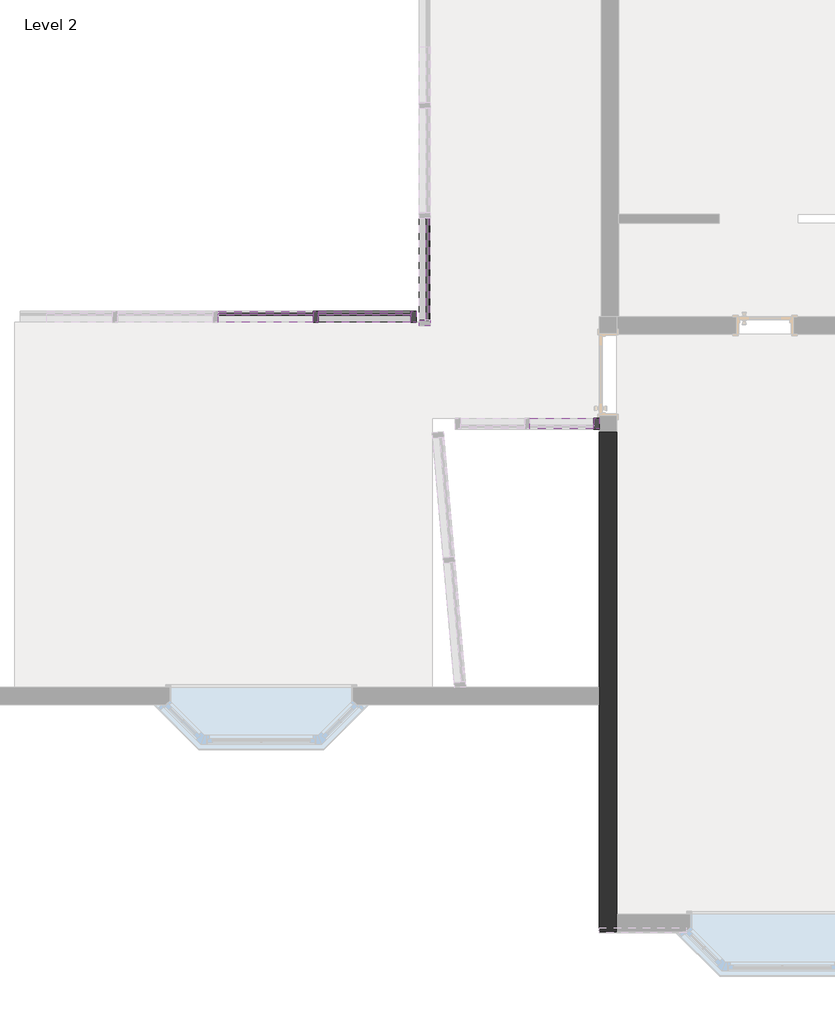
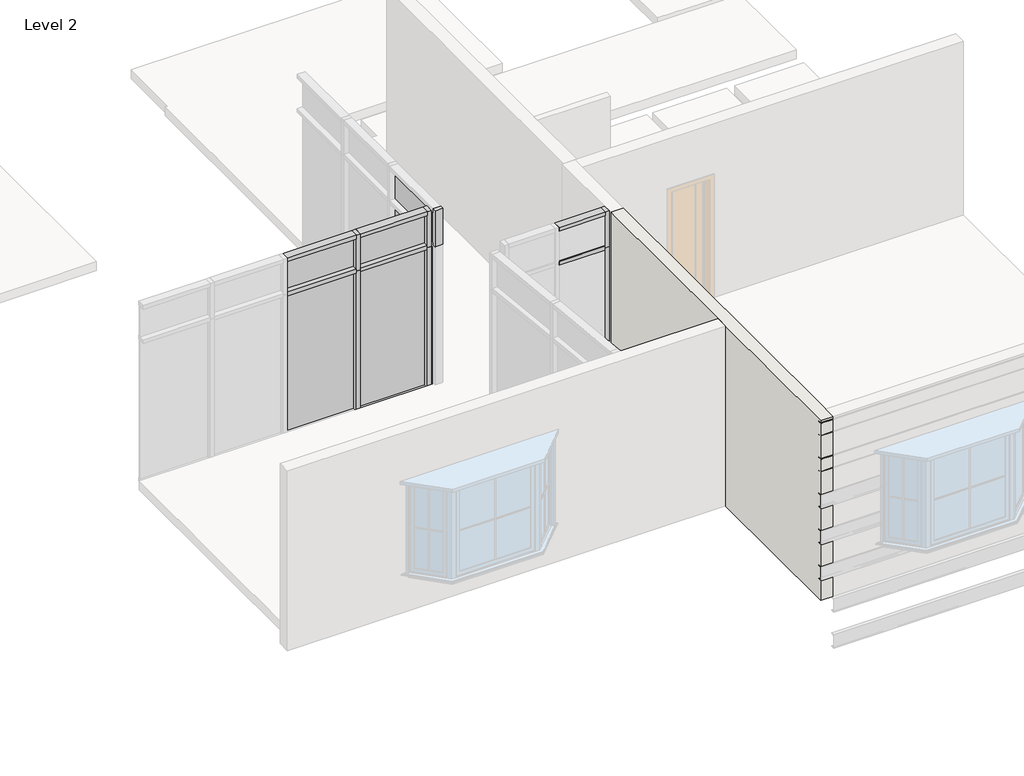
# One storey, part 3 of 5: 15 members, 6 plates, 1 wall.
"""IFC4 building model written with IfcOpenShell, lengths in millimetres."""

from ifc_helpers import new_model, si_unit, frame, origin, place, context, project, spatial, polyline, circle_curve, transform, mapped, element, save
from ifc_brep_helpers import plane_surface, cylinder_surface, revolved_surface, advanced_brep
from components import member_47bfaf8a, member_ee409385, member_0e454ba5, member_0d004d8a, member_f5e9651f, member_be44f791, member_766f1680, member_f0fea5a5, member_6e77e263, member_3a0a7659, member_7b995701, system_panel_glazed_d0e49211, system_panel_glazed_1bdee89b, system_panel_glazed_2e981f09, system_panel_glazed_87980334, system_panel_glazed_ed20128f, system_panel_glazed_d57d3c71

model = new_model("IFC4")

# Units and contexts
model_context = context("Model", 3, world=origin())
ifc_project = project(units=[si_unit("LENGTHUNIT", "METRE", prefix="MILLI")], contexts=[model_context])

# Site, building, storey
site = spatial("IfcSite", under=ifc_project)
building = spatial("IfcBuilding", under=site)
storey = spatial("IfcBuildingStorey", under=building, Name="Level 2", Elevation=3048.0)

# Members
placement = place(None, origin())
member_shape = member_47bfaf8a(model_context)
element("IfcMember", 1, ObjectType="Rectangular Mullion : 2.5\" x 5\" rectangular", at=placement, inside=storey, context=model_context, shape_type="MappedRepresentation", body=[
    mapped(member_shape, transform((-45780.9380314, -2939.8913973, 6096.0), x_axis=(0.0, -1.0, 0.0), y_axis=(1.0, 0.0, 0.0), z_axis=(0.0, 0.0, 1.0))),
])
element("IfcMember", 2, ObjectType="Rectangular Mullion : 2.5\" x 5\" rectangular", at=placement, inside=storey, context=model_context, shape_type="MappedRepresentation", body=[
    mapped(member_shape, transform((-43748.9380314, -4081.0930974, 5486.4), x_axis=(1.0, 0.0, 0.0), y_axis=(0.0, -1.0, 0.0), z_axis=(0.0, 0.0, -1.0))),
])
member_2_shape = member_ee409385(model_context)
element("IfcMember", 3, ObjectType="Rectangular Mullion : 2.5\" x 5\" rectangular", at=placement, inside=storey, context=model_context, shape_type="MappedRepresentation", body=[
    mapped(member_2_shape, transform((-43748.9380314, -4081.0930974, 3048.0), x_axis=(1.0, 0.0, 0.0), y_axis=(0.0, -1.0, 0.0), z_axis=(0.0, 0.0, -1.0))),
])
element("IfcMember", 4, ObjectType="Rectangular Mullion : 2.5\" x 5\" rectangular", at=placement, inside=storey, context=model_context, shape_type="MappedRepresentation", body=[
    mapped(member_2_shape, transform((-45882.5380314, -2838.2913973, 3048.0), x_axis=(1.0, 0.0, 0.0), y_axis=(0.0, -1.0, 0.0), z_axis=(0.0, 0.0, -1.0))),
])
element("IfcMember", 5, ObjectType="Rectangular Mullion : 2.5\" x 5\" rectangular", at=placement, inside=storey, context=model_context, shape_type="MappedRepresentation", body=[
    mapped(member_shape, transform((-45882.5380314, -2838.2913973, 5486.4), x_axis=(1.0, 0.0, 0.0), y_axis=(0.0, -1.0, 0.0), z_axis=(0.0, 0.0, -1.0))),
])
member_3_shape = member_0e454ba5(model_context)
element("IfcMember", 6, ObjectType="Rectangular Mullion : 2.5\" x 5\" rectangular", at=placement, inside=storey, context=model_context, shape_type="MappedRepresentation", body=[
    mapped(member_3_shape, transform((-45780.9380314, -2876.3913973, 3048.0), x_axis=(0.0, 0.0, -1.0), y_axis=(1.0, 0.0, 0.0), z_axis=(0.0, -1.0, 0.0))),
])
member_4_shape = member_0d004d8a(model_context)
element("IfcMember", 7, ObjectType="Rectangular Mullion : 2.5\" x 5\" rectangular", at=placement, inside=storey, context=model_context, shape_type="MappedRepresentation", body=[
    mapped(member_4_shape, transform((-45946.0380314, -2838.2913973, 6096.0), x_axis=(0.0, 0.0, 1.0), y_axis=(0.0, -1.0, 0.0), z_axis=(1.0, 0.0, 0.0))),
])
element("IfcMember", 8, ObjectType="Rectangular Mullion : 2.5\" x 5\" rectangular", at=placement, inside=storey, context=model_context, shape_type="MappedRepresentation", body=[
    mapped(member_4_shape, transform((-47019.1880316, -2838.2913973, 3048.0), x_axis=(0.0, 0.0, -1.0), y_axis=(0.0, -1.0, 0.0), z_axis=(-1.0, 0.0, 0.0))),
])
member_5_shape = member_f5e9651f(model_context)
element("IfcMember", 9, ObjectType="Rectangular Mullion : 2.5\" x 5\" rectangular", at=placement, inside=storey, context=model_context, shape_type="MappedRepresentation", body=[
    mapped(member_5_shape, transform((-47082.6880316, -2838.2913973, 6096.0), x_axis=(0.0, 0.0, 1.0), y_axis=(0.0, -1.0, 0.0), z_axis=(1.0, 0.0, 0.0))),
])
member_6_shape = member_be44f791(model_context)
element("IfcMember", 10, ObjectType="Rectangular Mullion : 2.5\" x 5\" rectangular", at=placement, inside=storey, context=model_context, shape_type="MappedRepresentation", body=[
    mapped(member_6_shape, transform((-45946.0380314, -2838.2913973, 5486.4), x_axis=(0.0, 0.0, 1.0), y_axis=(0.0, -1.0, 0.0), z_axis=(1.0, 0.0, 0.0))),
])
member_7_shape = member_766f1680(model_context)
element("IfcMember", 11, ObjectType="Rectangular Mullion : 2.5\" x 5\" rectangular", at=placement, inside=storey, context=model_context, shape_type="MappedRepresentation", body=[
    mapped(member_7_shape, transform((-47082.6880316, -2838.2913973, 5486.4), x_axis=(0.0, 0.0, 1.0), y_axis=(0.0, -1.0, 0.0), z_axis=(1.0, 0.0, 0.0))),
])
member_8_shape = member_f0fea5a5(model_context)
element("IfcMember", 12, ObjectType="Rectangular Mullion : 2.5\" x 5\" rectangular", at=placement, inside=storey, context=model_context, shape_type="MappedRepresentation", body=[
    mapped(member_8_shape, transform((-47050.9380316, -2838.2913973, 3048.0), x_axis=(1.0, 0.0, 0.0), y_axis=(0.0, -1.0, 0.0), z_axis=(0.0, 0.0, -1.0))),
])
member_9_shape = member_6e77e263(model_context)
element("IfcMember", 13, ObjectType="Rectangular Mullion : 2.5\" x 5\" rectangular", at=placement, inside=storey, context=model_context, shape_type="MappedRepresentation", body=[
    mapped(member_9_shape, transform((-47050.9380316, -2838.2913973, 5486.4), x_axis=(1.0, 0.0, 0.0), y_axis=(0.0, -1.0, 0.0), z_axis=(0.0, 0.0, -1.0))),
])
member_10_shape = member_3a0a7659(model_context)
element("IfcMember", 14, ObjectType="Rectangular Mullion : 2.5\" x 5\" rectangular", at=placement, inside=storey, context=model_context, shape_type="MappedRepresentation", body=[
    mapped(member_10_shape, transform((-43812.4380314, -4081.0930974, 6096.0), x_axis=(0.0, 0.0, 1.0), y_axis=(0.0, -1.0, 0.0), z_axis=(1.0, 0.0, 0.0))),
])
member_11_shape = member_7b995701(model_context)
element("IfcMember", 15, ObjectType="Rectangular Mullion : 2.5\" x 5\" rectangular", at=placement, inside=storey, context=model_context, shape_type="MappedRepresentation", body=[
    mapped(member_11_shape, transform((-43812.4380314, -4081.0930974, 5486.4), x_axis=(0.0, 0.0, 1.0), y_axis=(0.0, -1.0, 0.0), z_axis=(1.0, 0.0, 0.0))),
])

# Plates
system_panel_glazed_shape = system_panel_glazed_d0e49211(model_context)
element("IfcPlate", 16, ObjectType="System Panel : Glazed", at=placement, inside=storey, context=model_context, shape_type="MappedRepresentation", body=[
    mapped(system_panel_glazed_shape, transform((-45780.9380314, -2282.6663972, 3111.5), x_axis=(0.0, 1.0, 0.0), y_axis=(-1.0, 0.0, 0.0), z_axis=(0.0, 0.0, 1.0))),
])
system_panel_glazed_2_shape = system_panel_glazed_1bdee89b(model_context)
element("IfcPlate", 17, ObjectType="System Panel : Glazed", at=placement, inside=storey, context=model_context, shape_type="MappedRepresentation", body=[
    mapped(system_panel_glazed_2_shape, transform((-45780.9380314, -2282.6663972, 5518.15), x_axis=(0.0, 1.0, 0.0), y_axis=(-1.0, 0.0, 0.0), z_axis=(0.0, 0.0, 1.0))),
])
system_panel_glazed_3_shape = system_panel_glazed_2e981f09(model_context)
element("IfcPlate", 18, ObjectType="System Panel : Glazed", at=placement, inside=storey, context=model_context, shape_type="MappedRepresentation", body=[
    mapped(system_panel_glazed_3_shape, transform((-46482.6130315, -2838.2913973, 3111.5), x_axis=(1.0, 0.0, 0.0), y_axis=(0.0, 1.0, 0.0), z_axis=(0.0, 0.0, 1.0))),
])
system_panel_glazed_4_shape = system_panel_glazed_87980334(model_context)
element("IfcPlate", 19, ObjectType="System Panel : Glazed", at=placement, inside=storey, context=model_context, shape_type="MappedRepresentation", body=[
    mapped(system_panel_glazed_4_shape, transform((-47635.1380315, -2838.2913973, 3111.5), x_axis=(1.0, 0.0, 0.0), y_axis=(0.0, 1.0, 0.0), z_axis=(0.0, 0.0, 1.0))),
])
system_panel_glazed_5_shape = system_panel_glazed_ed20128f(model_context)
element("IfcPlate", 20, ObjectType="System Panel : Glazed", at=placement, inside=storey, context=model_context, shape_type="MappedRepresentation", body=[
    mapped(system_panel_glazed_5_shape, transform((-46482.6130315, -2838.2913973, 5518.15), x_axis=(1.0, 0.0, 0.0), y_axis=(0.0, 1.0, 0.0), z_axis=(0.0, 0.0, 1.0))),
])
system_panel_glazed_6_shape = system_panel_glazed_d57d3c71(model_context)
element("IfcPlate", 21, ObjectType="System Panel : Glazed", at=placement, inside=storey, context=model_context, shape_type="MappedRepresentation", body=[
    mapped(system_panel_glazed_6_shape, transform((-47635.1380315, -2838.2913973, 5518.15), x_axis=(1.0, 0.0, 0.0), y_axis=(0.0, 1.0, 0.0), z_axis=(0.0, 0.0, 1.0))),
])

# Wall
element("IfcWall", 22, ObjectType="OUTER WALL 8\"", at=placement, inside=storey, context=model_context, shape_type="AdvancedBrep", body=[
    advanced_brep(
    [(-43748.9380314, -4182.6930974, 3048.0), (-43748.9380314, -7156.2913973, 3048.0), (-43748.9380314, -7359.4913973, 3048.0), (-43748.9380314, -10001.0913973, 3048.0), (-43748.9380314, -10001.0913973, 3390.9), (-43748.9380314, -9952.7297973, 3390.9), (-43748.9380314, -9952.7297973, 3392.2796758), (-43748.9380314, -9957.1126065, 3397.4534103), (-43748.9380314, -9980.7332973, 3401.3902), (-43748.9380314, -9999.9711789, 3404.59652), (-43748.9380314, -10001.0913973, 3404.84689), (-43748.9380314, -10001.0913973, 3605.55311), (-43748.9380314, -9999.9711789, 3605.80348), (-43748.9380314, -9980.7332973, 3609.0098), (-43748.9380314, -9957.1126065, 3612.9465897), (-43748.9380314, -9952.7297973, 3618.1203242), (-43748.9380314, -9952.7297973, 3619.5), (-43748.9380314, -10001.0913973, 3619.5), (-43748.9380314, -10001.0913973, 4000.5), (-43748.9380314, -9952.7297973, 4000.5), (-43748.9380314, -9952.7297973, 4001.8796758), (-43748.9380314, -9957.1126065, 4007.0534103), (-43748.9380314, -9980.7332973, 4010.9902), (-43748.9380314, -9999.9711789, 4014.19652), (-43748.9380314, -10001.0913973, 4014.44689), (-43748.9380314, -10001.0913973, 4215.15311), (-43748.9380314, -9999.9711789, 4215.40348), (-43748.9380314, -9980.7332973, 4218.6098), (-43748.9380314, -9957.1126065, 4222.5465897), (-43748.9380314, -9952.7297973, 4227.7203242), (-43748.9380314, -9952.7297973, 4229.1), (-43748.9380314, -10001.0913973, 4229.1), (-43748.9380314, -10001.0913973, 4610.1), (-43748.9380314, -9952.7297973, 4610.1), (-43748.9380314, -9952.7297973, 4611.4796758), (-43748.9380314, -9957.1126065, 4616.6534103), (-43748.9380314, -9980.7332973, 4620.5902), (-43748.9380314, -9999.9711789, 4623.79652), (-43748.9380314, -10001.0913973, 4624.04689), (-43748.9380314, -10001.0913973, 4824.75311), (-43748.9380314, -9999.9711789, 4825.00348), (-43748.9380314, -9980.7332973, 4828.2098), (-43748.9380314, -9957.1126065, 4832.1465897), (-43748.9380314, -9952.7297973, 4837.3203242), (-43748.9380314, -9952.7297973, 4838.7), (-43748.9380314, -10001.0913973, 4838.7), (-43748.9380314, -10001.0913973, 5219.7), (-43748.9380314, -9952.7297973, 5219.7), (-43748.9380314, -9952.7297973, 5221.0796758), (-43748.9380314, -9957.1126065, 5226.2534103), (-43748.9380314, -9980.7332973, 5230.1902), (-43748.9380314, -9999.9711789, 5233.39652), (-43748.9380314, -10001.0913973, 5233.64689), (-43748.9380314, -10001.0913973, 5434.35311), (-43748.9380314, -9999.9711789, 5434.60348), (-43748.9380314, -9980.7332973, 5437.8098), (-43748.9380314, -9957.1126065, 5441.7465897), (-43748.9380314, -9952.7297973, 5446.9203242), (-43748.9380314, -9952.7297973, 5448.3), (-43748.9380314, -10001.0913973, 5448.3), (-43748.9380314, -10001.0913973, 5829.3), (-43748.9380314, -9952.7297973, 5829.3), (-43748.9380314, -9952.7297973, 5830.6796758), (-43748.9380314, -9957.1126065, 5835.8534103), (-43748.9380314, -9980.7332973, 5839.7902), (-43748.9380314, -9999.9711789, 5842.99652), (-43748.9380314, -10001.0913973, 5843.24689), (-43748.9380314, -10001.0913973, 6043.95311), (-43748.9380314, -9999.9711789, 6044.20348), (-43748.9380314, -9980.7332973, 6047.4098), (-43748.9380314, -9957.1126065, 6051.3465897), (-43748.9380314, -9952.7297973, 6056.5203242), (-43748.9380314, -9952.7297973, 6057.9), (-43748.9380314, -10001.0913973, 6057.9), (-43748.9380314, -10001.0913973, 6096.0), (-43748.9380314, -7359.4913973, 6096.0), (-43748.9380314, -7156.2913973, 6096.0), (-43748.9380314, -4182.6930974, 6096.0), (-43545.7380314, -10001.0913973, 3048.0), (-43545.7380314, -9797.8913973, 3048.0), (-43545.7380314, -4182.6930974, 3048.0), (-43545.7380314, -4182.6930974, 6096.0), (-43545.7380314, -9797.8913973, 6096.0), (-43545.7380314, -10001.0913973, 6096.0), (-43545.7380314, -10001.0913973, 6057.9), (-43545.7380314, -9952.7297973, 6057.9), (-43545.7380314, -9952.7297973, 6056.5203242), (-43545.7380314, -9957.1126065, 6051.3465897), (-43545.7380314, -9980.7332973, 6047.4098), (-43545.7380314, -9999.9711789, 6044.20348), (-43545.7380314, -10001.0913973, 6043.95311), (-43545.7380314, -10001.0913973, 5843.24689), (-43545.7380314, -9999.9711789, 5842.99652), (-43545.7380314, -9980.7332973, 5839.7902), (-43545.7380314, -9957.1126065, 5835.8534103), (-43545.7380314, -9952.7297973, 5830.6796758), (-43545.7380314, -9952.7297973, 5829.3), (-43545.7380314, -10001.0913973, 5829.3), (-43545.7380314, -10001.0913973, 5448.3), (-43545.7380314, -9952.7297973, 5448.3), (-43545.7380314, -9952.7297973, 5446.9203242), (-43545.7380314, -9957.1126065, 5441.7465897), (-43545.7380314, -9980.7332973, 5437.8098), (-43545.7380314, -9999.9711789, 5434.60348), (-43545.7380314, -10001.0913973, 5434.35311), (-43545.7380314, -10001.0913973, 5233.64689), (-43545.7380314, -9999.9711789, 5233.39652), (-43545.7380314, -9980.7332973, 5230.1902), (-43545.7380314, -9957.1126065, 5226.2534103), (-43545.7380314, -9952.7297973, 5221.0796758), (-43545.7380314, -9952.7297973, 5219.7), (-43545.7380314, -10001.0913973, 5219.7), (-43545.7380314, -10001.0913973, 4838.7), (-43545.7380314, -9952.7297973, 4838.7), (-43545.7380314, -9952.7297973, 4837.3203242), (-43545.7380314, -9957.1126065, 4832.1465897), (-43545.7380314, -9980.7332973, 4828.2098), (-43545.7380314, -9999.9711789, 4825.00348), (-43545.7380314, -10001.0913973, 4824.75311), (-43545.7380314, -10001.0913973, 4624.04689), (-43545.7380314, -9999.9711789, 4623.79652), (-43545.7380314, -9980.7332973, 4620.5902), (-43545.7380314, -9957.1126065, 4616.6534103), (-43545.7380314, -9952.7297973, 4611.4796758), (-43545.7380314, -9952.7297973, 4610.1), (-43545.7380314, -10001.0913973, 4610.1), (-43545.7380314, -10001.0913973, 4229.1), (-43545.7380314, -9952.7297973, 4229.1), (-43545.7380314, -9952.7297973, 4227.7203242), (-43545.7380314, -9957.1126065, 4222.5465897), (-43545.7380314, -9980.7332973, 4218.6098), (-43545.7380314, -9999.9711789, 4215.40348), (-43545.7380314, -10001.0913973, 4215.15311), (-43545.7380314, -10001.0913973, 4014.44689), (-43545.7380314, -9999.9711789, 4014.19652), (-43545.7380314, -9980.7332973, 4010.9902), (-43545.7380314, -9957.1126065, 4007.0534103), (-43545.7380314, -9952.7297973, 4001.8796758), (-43545.7380314, -9952.7297973, 4000.5), (-43545.7380314, -10001.0913973, 4000.5), (-43545.7380314, -10001.0913973, 3619.5), (-43545.7380314, -9952.7297973, 3619.5), (-43545.7380314, -9952.7297973, 3618.1203242), (-43545.7380314, -9957.1126065, 3612.9465897), (-43545.7380314, -9980.7332973, 3609.0098), (-43545.7380314, -9999.9711789, 3605.80348), (-43545.7380314, -10001.0913973, 3605.55311), (-43545.7380314, -10001.0913973, 3404.84689), (-43545.7380314, -9999.9711789, 3404.59652), (-43545.7380314, -9980.7332973, 3401.3902), (-43545.7380314, -9957.1126065, 3397.4534103), (-43545.7380314, -9952.7297973, 3392.2796758), (-43545.7380314, -9952.7297973, 3390.9), (-43545.7380314, -10001.0913973, 3390.9)],
    [
        (0, 1),
        (1, 2),
        (2, 3),
        (3, 4),
        (4, 5),
        (5, 6),
        (6, 7, circle_curve(frame((-43748.9380314, -9957.9748973, 3392.2796758), z_axis=(1.0, 0.0, 0.0), x_axis=(0.0, 1.0, 0.0)), 5.2451)),
        (7, 8),
        (8, 9),
        (9, 10, circle_curve(frame((-43748.9380314, -9998.2465973, 3414.943989), z_axis=(-1.0, 0.0, 0.0), x_axis=(0.0, 1.0, 0.0)), 10.4902)),
        (10, 11),
        (11, 12, circle_curve(frame((-43748.9380314, -9998.2465973, 3595.456011), z_axis=(-1.0, 0.0, 0.0), x_axis=(0.0, 1.0, 0.0)), 10.4902)),
        (12, 13),
        (13, 14),
        (14, 15, circle_curve(frame((-43748.9380314, -9957.9748973, 3618.1203242), z_axis=(1.0, 0.0, 0.0), x_axis=(0.0, 1.0, 0.0)), 5.2451)),
        (15, 16),
        (16, 17),
        (17, 18),
        (18, 19),
        (19, 20),
        (20, 21, circle_curve(frame((-43748.9380314, -9957.9748973, 4001.8796758), z_axis=(1.0, 0.0, 0.0), x_axis=(0.0, 1.0, 0.0)), 5.2451)),
        (21, 22),
        (22, 23),
        (23, 24, circle_curve(frame((-43748.9380314, -9998.2465973, 4024.543989), z_axis=(-1.0, 0.0, 0.0), x_axis=(0.0, 1.0, 0.0)), 10.4902)),
        (24, 25),
        (25, 26, circle_curve(frame((-43748.9380314, -9998.2465973, 4205.056011), z_axis=(-1.0, 0.0, 0.0), x_axis=(0.0, 1.0, 0.0)), 10.4902)),
        (26, 27),
        (27, 28),
        (28, 29, circle_curve(frame((-43748.9380314, -9957.9748973, 4227.7203242), z_axis=(1.0, 0.0, 0.0), x_axis=(0.0, 1.0, 0.0)), 5.2451)),
        (29, 30),
        (30, 31),
        (31, 32),
        (32, 33),
        (33, 34),
        (34, 35, circle_curve(frame((-43748.9380314, -9957.9748973, 4611.4796758), z_axis=(1.0, 0.0, 0.0), x_axis=(0.0, 1.0, 0.0)), 5.2451)),
        (35, 36),
        (36, 37),
        (37, 38, circle_curve(frame((-43748.9380314, -9998.2465973, 4634.143989), z_axis=(-1.0, 0.0, 0.0), x_axis=(0.0, 1.0, 0.0)), 10.4902)),
        (38, 39),
        (39, 40, circle_curve(frame((-43748.9380314, -9998.2465973, 4814.656011), z_axis=(-1.0, 0.0, 0.0), x_axis=(0.0, 1.0, 0.0)), 10.4902)),
        (40, 41),
        (41, 42),
        (42, 43, circle_curve(frame((-43748.9380314, -9957.9748973, 4837.3203242), z_axis=(1.0, 0.0, 0.0), x_axis=(0.0, 1.0, 0.0)), 5.2451)),
        (43, 44),
        (44, 45),
        (45, 46),
        (46, 47),
        (47, 48),
        (48, 49, circle_curve(frame((-43748.9380314, -9957.9748973, 5221.0796758), z_axis=(1.0, 0.0, 0.0), x_axis=(0.0, 1.0, 0.0)), 5.2451)),
        (49, 50),
        (50, 51),
        (51, 52, circle_curve(frame((-43748.9380314, -9998.2465973, 5243.743989), z_axis=(-1.0, 0.0, 0.0), x_axis=(0.0, 1.0, 0.0)), 10.4902)),
        (52, 53),
        (53, 54, circle_curve(frame((-43748.9380314, -9998.2465973, 5424.256011), z_axis=(-1.0, 0.0, 0.0), x_axis=(0.0, 1.0, 0.0)), 10.4902)),
        (54, 55),
        (55, 56),
        (56, 57, circle_curve(frame((-43748.9380314, -9957.9748973, 5446.9203242), z_axis=(1.0, 0.0, 0.0), x_axis=(0.0, 1.0, 0.0)), 5.2451)),
        (57, 58),
        (58, 59),
        (59, 60),
        (60, 61),
        (61, 62),
        (62, 63, circle_curve(frame((-43748.9380314, -9957.9748973, 5830.6796758), z_axis=(1.0, 0.0, 0.0), x_axis=(0.0, 1.0, 0.0)), 5.2451)),
        (63, 64),
        (64, 65),
        (65, 66, circle_curve(frame((-43748.9380314, -9998.2465973, 5853.343989), z_axis=(-1.0, 0.0, 0.0), x_axis=(0.0, 1.0, 0.0)), 10.4902)),
        (66, 67),
        (67, 68, circle_curve(frame((-43748.9380314, -9998.2465973, 6033.856011), z_axis=(-1.0, 0.0, 0.0), x_axis=(0.0, 1.0, 0.0)), 10.4902)),
        (68, 69),
        (69, 70),
        (70, 71, circle_curve(frame((-43748.9380314, -9957.9748973, 6056.5203242), z_axis=(1.0, 0.0, 0.0), x_axis=(0.0, 1.0, 0.0)), 5.2451)),
        (71, 72),
        (72, 73),
        (73, 74),
        (74, 75),
        (75, 76),
        (76, 77),
        (77, 0),
        (78, 79),
        (79, 80),
        (80, 81),
        (81, 82),
        (82, 83),
        (83, 84),
        (84, 85),
        (85, 86),
        (86, 87, circle_curve(frame((-43545.7380314, -9957.9748973, 6056.5203242), z_axis=(-1.0, 0.0, 0.0), x_axis=(0.0, 1.0, 0.0)), 5.2451)),
        (87, 88),
        (88, 89),
        (89, 90, circle_curve(frame((-43545.7380314, -9998.2465973, 6033.856011), z_axis=(1.0, 0.0, 0.0), x_axis=(0.0, 1.0, 0.0)), 10.4902)),
        (90, 91),
        (91, 92, circle_curve(frame((-43545.7380314, -9998.2465973, 5853.343989), z_axis=(1.0, 0.0, 0.0), x_axis=(0.0, 1.0, 0.0)), 10.4902)),
        (92, 93),
        (93, 94),
        (94, 95, circle_curve(frame((-43545.7380314, -9957.9748973, 5830.6796758), z_axis=(-1.0, 0.0, 0.0), x_axis=(0.0, 1.0, 0.0)), 5.2451)),
        (95, 96),
        (96, 97),
        (97, 98),
        (98, 99),
        (99, 100),
        (100, 101, circle_curve(frame((-43545.7380314, -9957.9748973, 5446.9203242), z_axis=(-1.0, 0.0, 0.0), x_axis=(0.0, 1.0, 0.0)), 5.2451)),
        (101, 102),
        (102, 103),
        (103, 104, circle_curve(frame((-43545.7380314, -9998.2465973, 5424.256011), z_axis=(1.0, 0.0, 0.0), x_axis=(0.0, 1.0, 0.0)), 10.4902)),
        (104, 105),
        (105, 106, circle_curve(frame((-43545.7380314, -9998.2465973, 5243.743989), z_axis=(1.0, 0.0, 0.0), x_axis=(0.0, 1.0, 0.0)), 10.4902)),
        (106, 107),
        (107, 108),
        (108, 109, circle_curve(frame((-43545.7380314, -9957.9748973, 5221.0796758), z_axis=(-1.0, 0.0, 0.0), x_axis=(0.0, 1.0, 0.0)), 5.2451)),
        (109, 110),
        (110, 111),
        (111, 112),
        (112, 113),
        (113, 114),
        (114, 115, circle_curve(frame((-43545.7380314, -9957.9748973, 4837.3203242), z_axis=(-1.0, 0.0, 0.0), x_axis=(0.0, 1.0, 0.0)), 5.2451)),
        (115, 116),
        (116, 117),
        (117, 118, circle_curve(frame((-43545.7380314, -9998.2465973, 4814.656011), z_axis=(1.0, 0.0, 0.0), x_axis=(0.0, 1.0, 0.0)), 10.4902)),
        (118, 119),
        (119, 120, circle_curve(frame((-43545.7380314, -9998.2465973, 4634.143989), z_axis=(1.0, 0.0, 0.0), x_axis=(0.0, 1.0, 0.0)), 10.4902)),
        (120, 121),
        (121, 122),
        (122, 123, circle_curve(frame((-43545.7380314, -9957.9748973, 4611.4796758), z_axis=(-1.0, 0.0, 0.0), x_axis=(0.0, 1.0, 0.0)), 5.2451)),
        (123, 124),
        (124, 125),
        (125, 126),
        (126, 127),
        (127, 128),
        (128, 129, circle_curve(frame((-43545.7380314, -9957.9748973, 4227.7203242), z_axis=(-1.0, 0.0, 0.0), x_axis=(0.0, 1.0, 0.0)), 5.2451)),
        (129, 130),
        (130, 131),
        (131, 132, circle_curve(frame((-43545.7380314, -9998.2465973, 4205.056011), z_axis=(1.0, 0.0, 0.0), x_axis=(0.0, 1.0, 0.0)), 10.4902)),
        (132, 133),
        (133, 134, circle_curve(frame((-43545.7380314, -9998.2465973, 4024.543989), z_axis=(1.0, 0.0, 0.0), x_axis=(0.0, 1.0, 0.0)), 10.4902)),
        (134, 135),
        (135, 136),
        (136, 137, circle_curve(frame((-43545.7380314, -9957.9748973, 4001.8796758), z_axis=(-1.0, 0.0, 0.0), x_axis=(0.0, 1.0, 0.0)), 5.2451)),
        (137, 138),
        (138, 139),
        (139, 140),
        (140, 141),
        (141, 142),
        (142, 143, circle_curve(frame((-43545.7380314, -9957.9748973, 3618.1203242), z_axis=(-1.0, 0.0, 0.0), x_axis=(0.0, 1.0, 0.0)), 5.2451)),
        (143, 144),
        (144, 145),
        (145, 146, circle_curve(frame((-43545.7380314, -9998.2465973, 3595.456011), z_axis=(1.0, 0.0, 0.0), x_axis=(0.0, 1.0, 0.0)), 10.4902)),
        (146, 147),
        (147, 148, circle_curve(frame((-43545.7380314, -9998.2465973, 3414.943989), z_axis=(1.0, 0.0, 0.0), x_axis=(0.0, 1.0, 0.0)), 10.4902)),
        (148, 149),
        (149, 150),
        (150, 151, circle_curve(frame((-43545.7380314, -9957.9748973, 3392.2796758), z_axis=(-1.0, 0.0, 0.0), x_axis=(0.0, 1.0, 0.0)), 5.2451)),
        (151, 152),
        (152, 153),
        (153, 78),
        (0, 80),
        (78, 3),
        (74, 83),
        (81, 77),
        (153, 4),
        (73, 84),
        (10, 147),
        (146, 11),
        (17, 140),
        (139, 18),
        (24, 133),
        (132, 25),
        (31, 126),
        (125, 32),
        (66, 91),
        (90, 67),
        (97, 60),
        (59, 98),
        (52, 105),
        (104, 53),
        (111, 46),
        (45, 112),
        (38, 119),
        (118, 39),
        (16, 141),
        (15, 142),
        (14, 143),
        (13, 144),
        (12, 145),
        (9, 148),
        (8, 149),
        (7, 150),
        (6, 151),
        (5, 152),
        (30, 127),
        (29, 128),
        (28, 129),
        (27, 130),
        (26, 131),
        (23, 134),
        (22, 135),
        (21, 136),
        (20, 137),
        (19, 138),
        (72, 85),
        (71, 86),
        (70, 87),
        (69, 88),
        (68, 89),
        (65, 92),
        (64, 93),
        (63, 94),
        (62, 95),
        (61, 96),
        (58, 99),
        (57, 100),
        (56, 101),
        (55, 102),
        (54, 103),
        (51, 106),
        (50, 107),
        (49, 108),
        (48, 109),
        (47, 110),
        (44, 113),
        (43, 114),
        (42, 115),
        (41, 116),
        (40, 117),
        (37, 120),
        (36, 121),
        (35, 122),
        (34, 123),
        (33, 124),
    ],
    [
        plane_surface(frame((-43748.9380314, -4081.0930974, 3048.0), z_axis=(-1.0, 0.0, 0.0), x_axis=(0.0, -1.0, 0.0))),
        plane_surface(frame((-43545.7380314, -4081.0930974, 3048.0), z_axis=(1.0, 0.0, 0.0), x_axis=(0.0, 1.0, 0.0))),
        plane_surface(frame((-43748.9380314, -4182.6930974, 3048.0), z_axis=(0.0, 0.0, -1.0), x_axis=(1.0, 0.0, 0.0))),
        plane_surface(frame((-43748.9380314, -9899.4913973, 6096.0), z_axis=(0.0, 0.0, 1.0), x_axis=(1.0, 0.0, 0.0))),
        plane_surface(frame((-43748.9380314, -4182.6930974, 6096.0), z_axis=(0.0, 1.0, 0.0), x_axis=(1.0, 0.0, 0.0))),
        plane_surface(frame((-43748.9380314, -10001.0913973, 3048.0), z_axis=(0.0, -1.0, 0.0), x_axis=(1.0, 0.0, 0.0))),
        plane_surface(frame((-43748.9380314, -10015.9757973, 3619.5), z_axis=(0.0, 0.0, -1.0), x_axis=(1.0, 0.0, 0.0))),
        plane_surface(frame((-43748.9380314, -9952.7297973, 3619.5), z_axis=(0.0, -1.0, 0.0), x_axis=(1.0, 0.0, 0.0))),
        revolved_surface(polyline([(-43748.9380314, -9952.7297973, 3618.1203242), (-43545.7380314, -9952.7297973, 3618.1203242)]), (-43748.9380314, -9957.9748973, 3618.1203242), (-1.0, 0.0, 0.0)),
        plane_surface(frame((-43748.9380314, -9957.1126065, 3612.9465897), z_axis=(0.0, -0.16439930721687082, 0.9863938705135049), x_axis=(1.0, 0.0, 0.0))),
        plane_surface(frame((-43748.9380314, -9980.7332973, 3609.0098), z_axis=(0.0, -0.16439930721687146, 0.9863938705135048), x_axis=(1.0, 0.0, 0.0))),
        cylinder_surface(frame((-43748.9380314, -9998.2465973, 3595.456011), z_axis=(1.0, 0.0, 0.0), x_axis=(0.0, 1.0, 0.0)), 10.4902),
        cylinder_surface(frame((-43748.9380314, -9998.2465973, 3414.943989), z_axis=(1.0, 0.0, 0.0), x_axis=(0.0, 1.0, 0.0)), 10.4902),
        plane_surface(frame((-43748.9380314, -9999.9711789, 3404.59652), z_axis=(0.0, -0.1643993072168769, -0.9863938705135039), x_axis=(1.0, 0.0, 0.0))),
        plane_surface(frame((-43748.9380314, -9980.7332973, 3401.3902), z_axis=(0.0, -0.16439930721687793, -0.9863938705135037), x_axis=(1.0, 0.0, 0.0))),
        revolved_surface(polyline([(-43748.9380314, -9952.7297973, 3392.2796758), (-43545.7380314, -9952.7297973, 3392.2796758)]), (-43748.9380314, -9957.9748973, 3392.2796758), (-1.0, 0.0, 0.0)),
        plane_surface(frame((-43748.9380314, -9952.7297973, 3392.2796758), z_axis=(0.0, -1.0, 0.0), x_axis=(1.0, 0.0, 0.0))),
        plane_surface(frame((-43748.9380314, -9952.7297973, 3390.9), z_axis=(0.0, 0.0, 1.0), x_axis=(1.0, 0.0, 0.0))),
        plane_surface(frame((-43748.9380314, -10015.9757973, 4229.1), z_axis=(0.0, 0.0, -1.0), x_axis=(1.0, 0.0, 0.0))),
        plane_surface(frame((-43748.9380314, -9952.7297973, 4229.1), z_axis=(0.0, -1.0, 0.0), x_axis=(1.0, 0.0, 0.0))),
        revolved_surface(polyline([(-43748.9380314, -9952.7297973, 4227.7203242), (-43545.7380314, -9952.7297973, 4227.7203242)]), (-43748.9380314, -9957.9748973, 4227.7203242), (-1.0, 0.0, 0.0)),
        plane_surface(frame((-43748.9380314, -9957.1126065, 4222.5465897), z_axis=(0.0, -0.16439930721687082, 0.9863938705135049), x_axis=(1.0, 0.0, 0.0))),
        plane_surface(frame((-43748.9380314, -9980.7332973, 4218.6098), z_axis=(0.0, -0.16439930721687146, 0.9863938705135048), x_axis=(1.0, 0.0, 0.0))),
        cylinder_surface(frame((-43748.9380314, -9998.2465973, 4205.056011), z_axis=(1.0, 0.0, 0.0), x_axis=(0.0, 1.0, 0.0)), 10.4902),
        cylinder_surface(frame((-43748.9380314, -9998.2465973, 4024.543989), z_axis=(1.0, 0.0, 0.0), x_axis=(0.0, 1.0, 0.0)), 10.4902),
        plane_surface(frame((-43748.9380314, -9999.9711789, 4014.19652), z_axis=(0.0, -0.1643993072168769, -0.9863938705135039), x_axis=(1.0, 0.0, 0.0))),
        plane_surface(frame((-43748.9380314, -9980.7332973, 4010.9902), z_axis=(0.0, -0.16439930721687793, -0.9863938705135037), x_axis=(1.0, 0.0, 0.0))),
        revolved_surface(polyline([(-43748.9380314, -9952.7297973, 4001.8796758), (-43545.7380314, -9952.7297973, 4001.8796758)]), (-43748.9380314, -9957.9748973, 4001.8796758), (-1.0, 0.0, 0.0)),
        plane_surface(frame((-43748.9380314, -9952.7297973, 4001.8796758), z_axis=(0.0, -1.0, 0.0), x_axis=(1.0, 0.0, 0.0))),
        plane_surface(frame((-43748.9380314, -9952.7297973, 4000.5), z_axis=(0.0, 0.0, 1.0), x_axis=(1.0, 0.0, 0.0))),
        plane_surface(frame((-43748.9380314, -10015.9757973, 6057.9), z_axis=(0.0, 0.0, -1.0), x_axis=(1.0, 0.0, 0.0))),
        plane_surface(frame((-43748.9380314, -9952.7297973, 6057.9), z_axis=(0.0, -1.0, 0.0), x_axis=(1.0, 0.0, 0.0))),
        revolved_surface(polyline([(-43748.9380314, -9952.7297973, 6056.5203242), (-43545.7380314, -9952.7297973, 6056.5203242)]), (-43748.9380314, -9957.9748973, 6056.5203242), (-1.0, 0.0, 0.0)),
        plane_surface(frame((-43748.9380314, -9957.1126065, 6051.3465897), z_axis=(0.0, -0.16439930721687082, 0.9863938705135049), x_axis=(1.0, 0.0, 0.0))),
        plane_surface(frame((-43748.9380314, -9980.7332973, 6047.4098), z_axis=(0.0, -0.16439930721687146, 0.9863938705135048), x_axis=(1.0, 0.0, 0.0))),
        cylinder_surface(frame((-43748.9380314, -9998.2465973, 6033.856011), z_axis=(1.0, 0.0, 0.0), x_axis=(0.0, 1.0, 0.0)), 10.4902),
        cylinder_surface(frame((-43748.9380314, -9998.2465973, 5853.343989), z_axis=(1.0, 0.0, 0.0), x_axis=(0.0, 1.0, 0.0)), 10.4902),
        plane_surface(frame((-43748.9380314, -9999.9711789, 5842.99652), z_axis=(0.0, -0.1643993072168769, -0.9863938705135039), x_axis=(1.0, 0.0, 0.0))),
        plane_surface(frame((-43748.9380314, -9980.7332973, 5839.7902), z_axis=(0.0, -0.16439930721687793, -0.9863938705135037), x_axis=(1.0, 0.0, 0.0))),
        revolved_surface(polyline([(-43748.9380314, -9952.7297973, 5830.6796758), (-43545.7380314, -9952.7297973, 5830.6796758)]), (-43748.9380314, -9957.9748973, 5830.6796758), (-1.0, 0.0, 0.0)),
        plane_surface(frame((-43748.9380314, -9952.7297973, 5830.6796758), z_axis=(0.0, -1.0, 0.0), x_axis=(1.0, 0.0, 0.0))),
        plane_surface(frame((-43748.9380314, -9952.7297973, 5829.3), z_axis=(0.0, 0.0, 1.0), x_axis=(1.0, 0.0, 0.0))),
        plane_surface(frame((-43748.9380314, -10015.9757973, 5448.3), z_axis=(0.0, 0.0, -1.0), x_axis=(1.0, 0.0, 0.0))),
        plane_surface(frame((-43748.9380314, -9952.7297973, 5448.3), z_axis=(0.0, -1.0, 0.0), x_axis=(1.0, 0.0, 0.0))),
        revolved_surface(polyline([(-43748.9380314, -9952.7297973, 5446.9203242), (-43545.7380314, -9952.7297973, 5446.9203242)]), (-43748.9380314, -9957.9748973, 5446.9203242), (-1.0, 0.0, 0.0)),
        plane_surface(frame((-43748.9380314, -9957.1126065, 5441.7465897), z_axis=(0.0, -0.16439930721687082, 0.9863938705135049), x_axis=(1.0, 0.0, 0.0))),
        plane_surface(frame((-43748.9380314, -9980.7332973, 5437.8098), z_axis=(0.0, -0.16439930721687146, 0.9863938705135048), x_axis=(1.0, 0.0, 0.0))),
        cylinder_surface(frame((-43748.9380314, -9998.2465973, 5424.256011), z_axis=(1.0, 0.0, 0.0), x_axis=(0.0, 1.0, 0.0)), 10.4902),
        cylinder_surface(frame((-43748.9380314, -9998.2465973, 5243.743989), z_axis=(1.0, 0.0, 0.0), x_axis=(0.0, 1.0, 0.0)), 10.4902),
        plane_surface(frame((-43748.9380314, -9999.9711789, 5233.39652), z_axis=(0.0, -0.1643993072168769, -0.9863938705135039), x_axis=(1.0, 0.0, 0.0))),
        plane_surface(frame((-43748.9380314, -9980.7332973, 5230.1902), z_axis=(0.0, -0.16439930721687793, -0.9863938705135037), x_axis=(1.0, 0.0, 0.0))),
        revolved_surface(polyline([(-43748.9380314, -9952.7297973, 5221.0796758), (-43545.7380314, -9952.7297973, 5221.0796758)]), (-43748.9380314, -9957.9748973, 5221.0796758), (-1.0, 0.0, 0.0)),
        plane_surface(frame((-43748.9380314, -9952.7297973, 5221.0796758), z_axis=(0.0, -1.0, 0.0), x_axis=(1.0, 0.0, 0.0))),
        plane_surface(frame((-43748.9380314, -9952.7297973, 5219.7), z_axis=(0.0, 0.0, 1.0), x_axis=(1.0, 0.0, 0.0))),
        plane_surface(frame((-43748.9380314, -10015.9757973, 4838.7), z_axis=(0.0, 0.0, -1.0), x_axis=(1.0, 0.0, 0.0))),
        plane_surface(frame((-43748.9380314, -9952.7297973, 4838.7), z_axis=(0.0, -1.0, 0.0), x_axis=(1.0, 0.0, 0.0))),
        revolved_surface(polyline([(-43748.9380314, -9952.7297973, 4837.3203242), (-43545.7380314, -9952.7297973, 4837.3203242)]), (-43748.9380314, -9957.9748973, 4837.3203242), (-1.0, 0.0, 0.0)),
        plane_surface(frame((-43748.9380314, -9957.1126065, 4832.1465897), z_axis=(0.0, -0.16439930721687082, 0.9863938705135049), x_axis=(1.0, 0.0, 0.0))),
        plane_surface(frame((-43748.9380314, -9980.7332973, 4828.2098), z_axis=(0.0, -0.16439930721687146, 0.9863938705135048), x_axis=(1.0, 0.0, 0.0))),
        cylinder_surface(frame((-43748.9380314, -9998.2465973, 4814.656011), z_axis=(1.0, 0.0, 0.0), x_axis=(0.0, 1.0, 0.0)), 10.4902),
        cylinder_surface(frame((-43748.9380314, -9998.2465973, 4634.143989), z_axis=(1.0, 0.0, 0.0), x_axis=(0.0, 1.0, 0.0)), 10.4902),
        plane_surface(frame((-43748.9380314, -9999.9711789, 4623.79652), z_axis=(0.0, -0.1643993072168769, -0.9863938705135039), x_axis=(1.0, 0.0, 0.0))),
        plane_surface(frame((-43748.9380314, -9980.7332973, 4620.5902), z_axis=(0.0, -0.16439930721687793, -0.9863938705135037), x_axis=(1.0, 0.0, 0.0))),
        revolved_surface(polyline([(-43748.9380314, -9952.7297973, 4611.4796758), (-43545.7380314, -9952.7297973, 4611.4796758)]), (-43748.9380314, -9957.9748973, 4611.4796758), (-1.0, 0.0, 0.0)),
        plane_surface(frame((-43748.9380314, -9952.7297973, 4611.4796758), z_axis=(0.0, -1.0, 0.0), x_axis=(1.0, 0.0, 0.0))),
        plane_surface(frame((-43748.9380314, -9952.7297973, 4610.1), z_axis=(0.0, 0.0, 1.0), x_axis=(1.0, 0.0, 0.0))),
    ],
    [
        (0, [[1, 2, 3, 4, 5, 6, 7, 8, 9, 10, 11, 12, 13, 14, 15, 16, 17, 18, 19, 20, 21, 22, 23, 24, 25, 26, 27, 28, 29, 30, 31, 32, 33, 34, 35, 36, 37, 38, 39, 40, 41, 42, 43, 44, 45, 46, 47, 48, 49, 50, 51, 52, 53, 54, 55, 56, 57, 58, 59, 60, 61, 62, 63, 64, 65, 66, 67, 68, 69, 70, 71, 72, 73, 74, 75, 76, 77, 78]]),
        (1, [[79, 80, 81, 82, 83, 84, 85, 86, 87, 88, 89, 90, 91, 92, 93, 94, 95, 96, 97, 98, 99, 100, 101, 102, 103, 104, 105, 106, 107, 108, 109, 110, 111, 112, 113, 114, 115, 116, 117, 118, 119, 120, 121, 122, 123, 124, 125, 126, 127, 128, 129, 130, 131, 132, 133, 134, 135, 136, 137, 138, 139, 140, 141, 142, 143, 144, 145, 146, 147, 148, 149, 150, 151, 152, 153, 154]]),
        (2, [[-3, -2, -1, 155, -80, -79, 156]]),
        (3, [[-77, -76, -75, 157, -83, -82, 158]]),
        (4, [[-78, -158, -81, -155]]),
        (5, [[-156, -154, 159, -4]]),
        (5, [[-157, -74, 160, -84]]),
        (5, [[-11, 161, -147, 162]]),
        (5, [[163, -140, 164, -18]]),
        (5, [[-25, 165, -133, 166]]),
        (5, [[167, -126, 168, -32]]),
        (5, [[-67, 169, -91, 170]]),
        (5, [[171, -60, 172, -98]]),
        (5, [[-53, 173, -105, 174]]),
        (5, [[175, -46, 176, -112]]),
        (5, [[-39, 177, -119, 178]]),
        (6, [[179, -141, -163, -17]]),
        (7, [[-179, -16, 180, -142]]),
        (8, [[-180, -15, 181, -143]]),
        (9, [[-181, -14, 182, -144]]),
        (10, [[-182, -13, 183, -145]]),
        (11, [[-183, -12, -162, -146]]),
        (12, [[184, -148, -161, -10]]),
        (13, [[-184, -9, 185, -149]]),
        (14, [[-185, -8, 186, -150]]),
        (15, [[-186, -7, 187, -151]]),
        (16, [[-187, -6, 188, -152]]),
        (17, [[-188, -5, -159, -153]]),
        (18, [[189, -127, -167, -31]]),
        (19, [[-189, -30, 190, -128]]),
        (20, [[-190, -29, 191, -129]]),
        (21, [[-191, -28, 192, -130]]),
        (22, [[-192, -27, 193, -131]]),
        (23, [[-193, -26, -166, -132]]),
        (24, [[194, -134, -165, -24]]),
        (25, [[-194, -23, 195, -135]]),
        (26, [[-195, -22, 196, -136]]),
        (27, [[-196, -21, 197, -137]]),
        (28, [[-197, -20, 198, -138]]),
        (29, [[-198, -19, -164, -139]]),
        (30, [[199, -85, -160, -73]]),
        (31, [[-199, -72, 200, -86]]),
        (32, [[-200, -71, 201, -87]]),
        (33, [[-201, -70, 202, -88]]),
        (34, [[-202, -69, 203, -89]]),
        (35, [[-203, -68, -170, -90]]),
        (36, [[204, -92, -169, -66]]),
        (37, [[-204, -65, 205, -93]]),
        (38, [[-205, -64, 206, -94]]),
        (39, [[-206, -63, 207, -95]]),
        (40, [[-207, -62, 208, -96]]),
        (41, [[-208, -61, -171, -97]]),
        (42, [[209, -99, -172, -59]]),
        (43, [[-209, -58, 210, -100]]),
        (44, [[-210, -57, 211, -101]]),
        (45, [[-211, -56, 212, -102]]),
        (46, [[-212, -55, 213, -103]]),
        (47, [[-213, -54, -174, -104]]),
        (48, [[214, -106, -173, -52]]),
        (49, [[-214, -51, 215, -107]]),
        (50, [[-215, -50, 216, -108]]),
        (51, [[-216, -49, 217, -109]]),
        (52, [[-217, -48, 218, -110]]),
        (53, [[-218, -47, -175, -111]]),
        (54, [[219, -113, -176, -45]]),
        (55, [[-219, -44, 220, -114]]),
        (56, [[-220, -43, 221, -115]]),
        (57, [[-221, -42, 222, -116]]),
        (58, [[-222, -41, 223, -117]]),
        (59, [[-223, -40, -178, -118]]),
        (60, [[224, -120, -177, -38]]),
        (61, [[-224, -37, 225, -121]]),
        (62, [[-225, -36, 226, -122]]),
        (63, [[-226, -35, 227, -123]]),
        (64, [[-227, -34, 228, -124]]),
        (65, [[-228, -33, -168, -125]]),
    ],
),
])

save(model, "model.ifc")

# Revit data of these elements
# Type "Rectangular Mullion : 2.5\" x 5\" rectangular"
#   built-in parameter 1007304 = 0.416667 (stored number, unit not read)
#   built-in parameter 1007301 = 0.104167 (stored number, unit not read)
#   built-in parameter 1007300 = 0.104167 (stored number, unit not read)
# Type "System Panel : Glazed"
#   Construction Type Id = "GSP4R"
#   Analytic Construction = "1/8 in Pilkington single glazing"
#   Visual Light Transmittance = 0.9
#   Solar Heat Gain Coefficient = 0.86
#   Heat Transfer Coefficient (U) = 1.18115 BTU/(h·ft²·°F)
#   Define Thermal Properties by = 1
# Type "OUTER WALL 8\""
#   Assembly Code = "B2010"
#   Layers, outside or top first: 0' - 8" "BEIGE COLOUR" (function 1)
# Elements 1, 2, 3, 4, 5, 6, 7, 8, 9, 10, 11, 12, 13, 14, 15 (IfcMember, "Rectangular Mullion : 2.5\" x 5\" rectangular")
#   Phase Created = New Construction
#   Materials on its faces: "Aluminum"
# Elements 16, 17, 18, 19, 20, 21 (IfcPlate, "System Panel : Glazed")
#   Phase Created = New Construction
#   Materials on its faces: "glass panel 223"
# Element 22 (IfcWall, "OUTER WALL 8\"")
#   Top Offset = 0' - 0"
#   Base Offset = 0' - 0"
#   wall height = 10' - 0"
#   Phase Created = New Construction
#   Base Constraint = Level 2
#   Top Constraint = Level 3
#   Materials on its faces: "BEIGE COLOUR"
# Materials
#   "BEIGE COLOUR": class "Generic", colour RGB 120 120 120, transparency 0, Cost = 0
#   "Aluminum": class "Metal", colour RGB 247 247 247, transparency 0, Description = "Aluminum 6061", Cost = 0
#   "glass panel 223": class "Generic", colour RGB 120 120 120, transparency 0, Cost = 0
